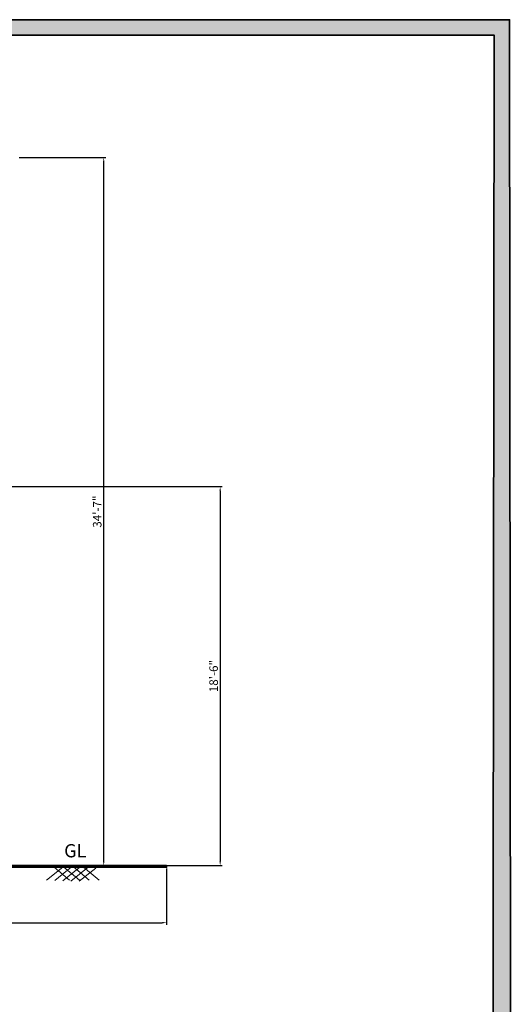
# Model space of a CAD drawing. Units: inches. Extents: x 1804 to 3296, y 909 to 2477.
# Tile 31 of 31: x 3008 to 3296, y 1900 to 2477. Entities that reach past the tile are written whole.
import ezdxf

# ---------------------------------------------------------------- set-up
doc = ezdxf.new("R2010")
doc.units = ezdxf.units.IN
for name, color, linetype, lineweight in [('A-ANNO-DIMS', 2, 'Continuous', 18), ('A-ANNO-TTLB', 156, 'Continuous', 35), ('A-SECT-PATT', 160, 'Continuous', 13), ('A-WALL-PATT', 10, 'Continuous', 13), ('C-GRAD-PATT', 8, 'Continuous', 13), ('SEC', 160, 'Continuous', 35), ('TEXT', 190, 'Continuous', 18)]:
    doc.layers.add(name, color=color, linetype=linetype, lineweight=lineweight)
doc.styles.get("Standard").update_dxf_attribs({"font": 'arial.ttf'})
doc.dimstyles.new('ISO-25', dxfattribs={"dimtxt": 5, "dimasz": 2.5, "dimexe": 1.25, "dimexo": 0.625, "dimtad": 1, "dimdec": 0, "dimlunit": 4, "dimtxsty": 'Standard', "dimcen": 2.5, "dimadec": 0, "dimazin": 0, "dimtfac": 1, "dimtdec": 0, "dimtmove": 0, "dimatfit": 3, "dimfxl": 1, "dimarcsym": 0})

# ---------------------------------------------------------------- blocks, each defined once
blk = doc.blocks.new('*D33')
at = {"layer": 'A-ANNO-DIMS', "color": 0, "lineweight": -2, "transparency": 16777216}
for p, q in [((3007.45, 2395.8), (3058.21, 2395.8)), ((3056.96, 1983.77), (3056.96, 2393.3)), ((3007.45, 1981.27), (3058.21, 1981.27))]:
    blk.add_line(p, q, dxfattribs=at)
at = {"layer": 'A-ANNO-DIMS', "color": 0, "lineweight": 100, "transparency": 16777216}
for points in [[(3056.55, 2393.3), (3057.38, 2393.3), (3056.96, 2395.8)], [(3056.55, 1983.77), (3057.38, 1983.77), (3056.96, 1981.27)]]:
    blk.add_solid(points, dxfattribs=at)
at = {"layer": 'Defpoints', "color": 0, "lineweight": 100, "transparency": 16777216}
for p in [(3006.82, 2395.8), (3056.96, 2395.8), (3006.82, 1981.27)]:
    blk.add_point(p, dxfattribs=at)
at = {"layer": 'A-ANNO-DIMS', "color": 0, "transparency": 16777216, "insert": (3053.79, 2188.53), "char_height": 5, "attachment_point": 5, "rotation": 90}
blk.add_mtext('34\'-7"', dxfattribs=at)
blk = doc.blocks.new('*D91')
at = {"layer": 'A-ANNO-DIMS', "color": 0, "lineweight": -2, "transparency": 16777216}
for p, q in [((2490.75, 1978.65), (2490.75, 1946.62)), ((3093.73, 1979.65), (3093.73, 1946.62)), ((2493.25, 1947.87), (3091.23, 1947.87))]:
    blk.add_line(p, q, dxfattribs=at)
at = {"layer": 'A-ANNO-DIMS', "color": 0, "lineweight": 100, "transparency": 16777216}
for points in [[(2493.25, 1948.29), (2493.25, 1947.46), (2490.75, 1947.87)], [(3091.23, 1948.29), (3091.23, 1947.46), (3093.73, 1947.87)]]:
    blk.add_solid(points, dxfattribs=at)
at = {"layer": 'Defpoints', "color": 0, "lineweight": 100, "transparency": 16777216}
for p in [(2490.75, 1979.27), (3093.73, 1980.27), (3093.73, 1947.87)]:
    blk.add_point(p, dxfattribs=at)
at = {"layer": 'A-ANNO-DIMS', "color": 0, "transparency": 16777216, "insert": (2792.24, 1951.05), "char_height": 5, "attachment_point": 5}
blk.add_mtext('50\'-3"', dxfattribs=at)
blk = doc.blocks.new('*D93')
at = {"layer": 'A-ANNO-DIMS', "color": 0, "lineweight": -2, "transparency": 16777216}
for p, q in [((2997.45, 2203.2), (3126.38, 2203.2)), ((3125.13, 2200.7), (3125.13, 1983.77)), ((3007.45, 1981.27), (3126.38, 1981.27))]:
    blk.add_line(p, q, dxfattribs=at)
at = {"layer": 'A-ANNO-DIMS', "color": 0, "lineweight": 100, "transparency": 16777216}
for points in [[(3124.71, 2200.7), (3125.55, 2200.7), (3125.13, 2203.2)], [(3124.71, 1983.77), (3125.55, 1983.77), (3125.13, 1981.27)]]:
    blk.add_solid(points, dxfattribs=at)
at = {"layer": 'Defpoints', "color": 0, "lineweight": 100, "transparency": 16777216}
for p in [(2996.82, 2203.2), (3006.82, 1981.27), (3125.13, 1981.27)]:
    blk.add_point(p, dxfattribs=at)
at = {"layer": 'A-ANNO-DIMS', "color": 0, "transparency": 16777216, "insert": (3121.95, 2092.24), "char_height": 5, "attachment_point": 5, "rotation": 90}
blk.add_mtext('18\'-6"', dxfattribs=at)

msp = doc.modelspace()

# ---------------------------------------------------------------- hatches: boundary and pattern name
at = {"layer": 'A-ANNO-TTLB'}
h = msp.add_hatch(color=256, dxfattribs=at)
h.dxf.hatch_style = 1
h.paths.add_polyline_path([(3294.53, 2476.54), (1803.79, 2476.54), (1805.43, 909.47), (3296.17, 909.47)])
h.paths.add_polyline_path([(1811, 914.33), (1812.79, 2467.54), (3285.53, 2467.54), (3283.74, 914.33)], flags=16)
h.paths.add_polyline_path([(1925.58, 1062.77), (1925.58, 1138.07), (1925.58, 1539.88), (1925.58, 1793.38), (1925.58, 1830.04), (2325.54, 1830.04), (2325.54, 1793.38), (2325.54, 1586.42), (2325.54, 1138.07), (2325.54, 1062.77)], flags=0)
h.paths.add_polyline_path([(1997.22, 1029.4), (2008.85, 1037.96), (2008.85, 1020.84)], flags=0)
h.paths.add_polyline_path([(1934.58, 1138.07), (1934.58, 1147.07), (2078.77, 1147.07), (2078.77, 1138.07), (2060.94, 1138.07)], flags=0)
h.paths.add_polyline_path([(1944.35, 1138.07), (1944.35, 1147.07), (2056.05, 1147.07), (2056.05, 1138.07)], flags=0)
h.paths.add_polyline_path([(2222.24, 1037.96), (2233.87, 1029.4), (2222.24, 1020.84)], flags=0)
h.paths.add_polyline_path([(2061.94, 1139.07), (2061.94, 1146.07), (2077.77, 1146.07), (2077.77, 1139.07)], flags=0)
h.paths.add_polyline_path([(2149.58, 1138.07), (2149.58, 1269.44), (2158.58, 1269.44), (2158.58, 1326.69), (2149.58, 1326.69), (2149.58, 1340.94), (2139.6, 1340.94), (2139.6, 1434.25), (2149.58, 1434.25), (2149.58, 1447.36), (2158.58, 1447.36), (2158.58, 1423.87), (2158.58, 1408.06), (2198.46, 1408.06), (2198.46, 1412.56), (2282.65, 1412.56), (2282.65, 1465.94), (2316.54, 1465.94), (2316.54, 1590.92), (2192.86, 1590.92), (2192.86, 1595.3), (2291.17, 1595.3), (2291.17, 1590.92), (2316.54, 1590.92), (2316.54, 1784.38), (2300.24, 1784.38), (2300.24, 1757.47), (2268, 1757.47), (2268, 1681.04), (2180.87, 1681.04), (2180.87, 1757.47), (2148.63, 1757.47), (2148.63, 1784.38), (2119.08, 1784.38), (2119.08, 1585.58), (2114.58, 1585.58), (2114.58, 1784.38), (2064.11, 1784.38), (2046.28, 1784.38), (2046.28, 1760.38), (1958.58, 1760.38), (1958.58, 1664.38), (1934.58, 1664.38), (1934.58, 1784.38), (1934.58, 1793.38), (2046.28, 1793.38), (2064.11, 1793.38), (2119.08, 1793.38), (2230.78, 1793.38), (2230.78, 1784.38), (2268, 1784.38), (2300.24, 1784.38), (2316.54, 1784.38), (2316.54, 1590.92), (2316.54, 1373.73), (2316.54, 1138.07)], flags=0)
h.paths.add_polyline_path([(2209.19, 1166.63), (2209.19, 1175.63), (2158.58, 1175.63), (2209.19, 1223.63), (2209.19, 1231.63), (2183.88, 1231.63), (2183.88, 1301.66), (2242.59, 1301.66), (2242.59, 1326.69), (2316.54, 1326.69), (2272.59, 1271.63), (2272.59, 1223.63), (2316.54, 1175.63), (2272.59, 1175.63), (2272.59, 1166.63)], flags=0)
h.paths.add_polyline_path([(1947.77, 1345.22), (1947.77, 1457.48), (1991.2, 1457.48), (1991.2, 1451.7), (1991.2, 1352.18), (1991.2, 1345.22)], flags=0)
h.paths.add_polyline_path([(2209.19, 1271.63), (2262.59, 1271.63), (2262.59, 1311.85), (2272.59, 1301.66), (2272.59, 1271.63), (2269.92, 1269.63), (2270.59, 1269.63), (2270.59, 1225.63), (2211.19, 1225.63), (2211.19, 1269.63), (2211.86, 1269.63)], flags=0)
h.paths.add_polyline_path([(2000.34, 1378.21), (2000.34, 1429.71), (2025.22, 1429.71), (2025.22, 1378.21)], flags=0)
h.paths.add_polyline_path([(2001.34, 1379.21), (2001.34, 1428.71), (2024.22, 1428.71), (2024.22, 1379.21)], flags=0)
h.paths.add_polyline_path([(2012.34, 1390.21), (2012.34, 1417.71), (2013.22, 1417.71), (2013.22, 1390.21)], flags=0)
h.paths.add_polyline_path([(2237.56, 1331.19), (2237.56, 1340.18), (2238.62, 1340.18), (2238.62, 1386.84), (2241.04, 1386.84), (2242.06, 1386.84), (2242.06, 1408.06), (2316.54, 1331.19)], flags=0)
h.paths.add_polyline_path([(1953.73, 1464.35), (1953.73, 1498.59), (1981.74, 1498.59), (1981.74, 1464.35)], flags=0)
h.paths.add_polyline_path([(1987.63, 1462.08), (1987.63, 1500.95), (2104.07, 1500.95), (2104.07, 1462.08), (2099.27, 1462.08), (1993.6, 1462.08)], flags=0)
h.paths.add_polyline_path([(1956.06, 1481.47, -1), (1979.41, 1481.47, -1)], flags=0)
edge = h.paths.add_edge_path(flags=0)
edge.add_ellipse((2299.53, 1438.37), major_axis=(0.31, 21.36), ratio=0.670333, start_angle=0, end_angle=360)
h.paths.add_polyline_path([(2297.39, 1438.37, -1), (2301.67, 1438.37, -1)], flags=0)
h.paths.add_polyline_path([(2591.54, 1163.23), (2591.54, 1179.38), (2591.54, 1379.68), (2591.54, 1395.84), (2734.5, 1395.84), (2734.5, 1379.68), (2734.5, 1179.38), (2734.5, 1163.23)], flags=0)
h.paths.add_polyline_path([(2592.54, 1164.23), (2592.54, 1166.23), (2733.5, 1166.23), (2733.5, 1164.23)], flags=0)
h.paths.add_polyline_path([(2592.54, 1180.38), (2592.54, 1378.68), (2733.5, 1378.68), (2733.5, 1180.38)], flags=0)
h.paths.add_polyline_path([(2593.54, 1181.38), (2593.54, 1377.68), (2732.5, 1377.68), (2732.5, 1181.38)], flags=0)
h.paths.add_polyline_path([(2594.54, 1182.38), (2594.54, 1376.68), (2731.5, 1376.68), (2731.5, 1182.38)], flags=0)
h.paths.add_polyline_path([(1936.95, 1697.46), (1936.95, 1736.46), (1955.41, 1736.46), (1955.41, 1697.46)], flags=0)
h.paths.add_polyline_path([(1938.48, 1718.36), (1938.48, 1734.92), (1953.65, 1734.92), (1953.65, 1718.36)], flags=0)
h.paths.add_polyline_path([(1944.75, 1726.64, -1), (1947.37, 1726.64, -1)], flags=0)
h.paths.add_polyline_path([(2592.54, 1394.84), (2733.5, 1394.84), (2733.5, 1392.84), (2592.54, 1392.84)], flags=0)
h.paths.add_polyline_path([(1976.61, 1762.5), (1976.61, 1781.44), (2012.79, 1781.44), (2012.79, 1762.5)], flags=0)
h.paths.add_polyline_path([(1979.57, 1771.97, -1), (1991.39, 1771.97, -1)], flags=0)
h.paths.add_polyline_path([(1995.36, 1771.97, -1), (2007.18, 1771.97, -1)], flags=0)
h.paths.add_polyline_path([(2251.51, 1744.53), (2268, 1730.05), (2251.51, 1730.05)], flags=0)
h.paths.add_polyline_path([(2047.28, 1785.38), (2047.28, 1792.38), (2063.11, 1792.38), (2063.11, 1785.38)], flags=0)
h.paths.add_polyline_path([(2155.08, 1770.92, -1), (2174.42, 1770.92, -1)], flags=0)
h.paths.add_polyline_path([(2188.59, 1758.27), (2188.59, 1772.81), (2222.3, 1772.81), (2222.3, 1758.27)], flags=0)
h.paths.add_polyline_path([(2223.97, 1758.27), (2223.97, 1772.81), (2257.68, 1772.81), (2257.68, 1758.27)], flags=0)
h.paths.add_polyline_path([(2274.45, 1770.92, -1), (2293.8, 1770.92, -1)], flags=0)
h.paths.add_polyline_path([(2591.54, 1582.09), (2591.54, 1782.39), (2734.5, 1782.39), (2734.5, 1582.09)], flags=0)
h.paths.add_polyline_path([(2592.54, 1583.09), (2592.54, 1781.39), (2733.5, 1781.39), (2733.5, 1583.09)], flags=0)
h.paths.add_polyline_path([(2593.54, 1584.09), (2593.54, 1780.39), (2732.5, 1780.39), (2732.5, 1584.09)], flags=0)
h.paths.add_polyline_path([(2594.54, 1585.09), (2594.54, 1779.39), (2731.5, 1779.39), (2731.5, 1585.09)], flags=0)
h.paths.add_polyline_path([(1922.17, 1978.79), (1922.17, 2295.08), (1922.17, 2296.08), (2115.67, 2296.08), (2115.67, 2384.31), (2115.67, 2385.31), (2322.12, 2385.31), (2323.12, 2385.31), (2323.12, 1979.79), (2323.12, 1978.79), (1923.17, 1978.79)], flags=0)
h.paths.add_polyline_path([(1922.17, 1978.79), (1922.17, 2051.31), (1922.17, 2214.86), (1922.17, 2296.08), (2115.67, 2296.08), (2115.67, 2385.31), (2323.12, 2385.31), (2323.12, 2280.42), (2323.12, 1978.79), (2115.67, 1978.79)], flags=0)
h.paths.add_polyline_path([(1923.17, 1979.79), (1923.17, 2050.31), (2115.67, 2050.31), (2115.67, 2051.31), (1923.17, 2051.31), (1923.17, 2213.86), (1923.17, 2214.86), (1923.17, 2295.08), (1990.02, 2295.08), (1990.02, 2214.86), (1991.02, 2214.86), (1991.02, 2295.08), (2115.67, 2295.08), (2115.67, 1979.79), (2116.67, 1979.79), (2116.67, 2304.18), (2116.67, 2384.31), (2322.12, 2384.31), (2322.12, 2280.42), (2322.12, 1979.79), (2115.67, 1979.79)], flags=0)
h.paths.add_polyline_path([(2972.46, 1192.5), (2972.46, 1196.92), (2995.47, 1196.92), (2995.47, 1255.47), (2995.09, 1255.47), (2987.42, 1249.39), (2980.08, 1255.47), (2978.05, 1255.47), (2978.05, 1257.24), (2995.47, 1257.24), (2995.47, 1261.58), (3015.37, 1261.58), (3015.37, 1333.28), (3015.37, 1414.4), (3032.82, 1414.4), (3032.82, 1333.28), (3032.82, 1261.58), (3052.66, 1261.58), (3052.66, 1255.47), (3079.86, 1255.47), (3078.72, 1254.57), (3081.47, 1252.29), (3078.56, 1249.99), (3075.81, 1252.26), (3072.57, 1249.69), (3070.36, 1251.52), (3067.67, 1249.39), (3060.34, 1255.47), (3052.66, 1255.47), (3052.66, 1196.92), (3054.58, 1196.92), (3074, 1196.92), (3074, 1192.5), (3052.66, 1192.5), (2995.47, 1192.5)], flags=0)
h.paths.add_polyline_path([(2490.75, 1979.27), (2490.75, 1980.27), (2596.87, 1980.27), (2596.87, 2051.8), (2596.87, 2052.8), (2596.87, 2216.35), (2596.87, 2297.57), (2717.32, 2297.57), (2710.57, 2305.62), (2724.07, 2305.62), (2717.32, 2297.57), (2782.37, 2297.57), (2782.37, 2395.8), (3006.82, 2395.8), (3006.82, 1981.27), (3093.73, 1981.27), (3093.73, 1980.27), (3047.51, 1980.27), (3046.37, 1979.37), (3049.11, 1977.1), (3046.2, 1974.79), (3043.46, 1977.07), (3040.21, 1974.49), (3038, 1976.32), (3035.32, 1974.2), (3027.98, 1980.27), (2871.83, 1980.27), (2871.83, 1981.27), (2791.37, 1981.27), (2791.37, 2050.8), (2597.87, 2050.8), (2597.87, 1980.27), (2597.87, 1979.27), (2546.27, 1979.27), (2545.12, 1978.37), (2547.87, 1976.1), (2544.96, 1973.79), (2542.22, 1976.07), (2538.97, 1973.49), (2536.76, 1975.32), (2534.07, 1973.2), (2526.74, 1979.27)], flags=0)
h.paths.add_polyline_path([(2597.87, 2051.8), (2606.87, 2051.8), (2606.87, 2258.39), (2597.87, 2258.39), (2597.87, 2296.57), (2606.87, 2296.57), (2606.87, 2262.39), (2782.37, 2262.39), (2782.37, 2296.57), (2790.37, 2296.57), (2790.37, 2262.39), (2791.37, 2262.39), (2791.37, 2305.67), (2791.37, 2385.8), (2996.82, 2385.8), (2996.82, 2339.85), (3006.82, 2339.85), (3006.82, 2250.12), (2997.82, 2250.12), (2997.82, 1981.27), (2996.82, 1981.27), (2872.83, 1981.27), (2872.83, 1991.8), (2871.83, 1991.8), (2871.83, 2050.8), (2790.37, 2050.8), (2597.87, 2050.8)], flags=0)
h.paths.add_polyline_path([(2179.93, 2153.92), (2179.93, 2353.97), (2259.98, 2353.97), (2259.98, 2153.92)], flags=0)
h.paths.add_polyline_path([(2180.93, 2154.92), (2180.93, 2352.97), (2258.98, 2352.97), (2258.98, 2154.92)], flags=0)
h.paths.add_polyline_path([(2960.87, 1608.49), (2960.87, 1753.62), (3070.9, 1753.62), (3070.9, 1608.49)], flags=0)
h.paths.add_polyline_path([(2961.87, 1609.49), (2961.87, 1752.62), (3069.9, 1752.62), (3069.9, 1609.49)], flags=0)
h.paths.add_polyline_path([(2962.87, 1610.49), (2962.87, 1751.62), (3068.9, 1751.62), (3068.9, 1610.49)], flags=0)
h.paths.add_polyline_path([(2963.87, 1611.49), (2963.87, 1750.62), (3067.9, 1750.62), (3067.9, 1611.49)], flags=0)
h.paths.add_polyline_path([(2782.37, 2051.8), (2782.37, 2216.32), (2791.37, 2216.32), (2791.37, 2051.8), (2872.83, 2051.8), (2872.83, 2068.56), (2884.67, 2068.56), (2884.67, 2085.33), (2896.51, 2085.33), (2896.51, 2102.09), (2908.36, 2102.09), (2908.36, 2118.85), (2920.2, 2118.85), (2920.2, 2135.62), (2932.05, 2135.62), (2932.05, 2145.3), (2925.08, 2145.3), (2925.08, 2203.2), (2996.82, 2203.2), (2996.82, 2145.3), (2953.82, 2145.3), (2872.83, 2051.8), (2790.37, 2051.8)], flags=0)
h.paths.add_polyline_path([(2717.32, 2238.65), (2710.57, 2246.7), (2724.07, 2246.7)], flags=0)
h.paths.add_polyline_path([(2003.09, 1122.79), (2017.16, 1122.79), (2017.16, 1138.74), (2003.09, 1138.74)], flags=8)
h.paths.add_polyline_path([(2174.76, 1792.72), (2188.83, 1792.72), (2188.83, 1808.66), (2174.76, 1808.66)], flags=8)
h.paths.add_polyline_path([(1987.95, 1792.51), (2002.02, 1792.51), (2002.02, 1808.45), (1987.95, 1808.45)], flags=8)
h.paths.add_polyline_path([(2148.79, 1289.26), (2160.46, 1289.26), (2160.46, 1305.2), (2148.79, 1305.2)], flags=8)
h.paths.add_polyline_path([(2115.36, 1133.57), (2127.04, 1133.57), (2127.04, 1149.51), (2115.36, 1149.51)], flags=8)
h.paths.add_polyline_path([(2237.58, 1421.48), (2249.25, 1421.48), (2249.25, 1437.43), (2237.58, 1437.43)], flags=8)
h.paths.add_polyline_path([(2134.99, 1584.32), (2146.66, 1584.32), (2146.66, 1600.26), (2134.99, 1600.26)], flags=8)
h.paths.add_polyline_path([(2101.95, 1557.31), (2113.62, 1557.31), (2113.62, 1573.25), (2101.95, 1573.25)], flags=8)
h.paths.add_polyline_path([(2937.85, 1156.77), (3120.41, 1156.77), (3120.41, 1185.72), (2937.85, 1185.72)], flags=8)
h.paths.add_polyline_path([(2980.71, 1786.71), (3050.06, 1786.71), (3050.06, 1802.66), (2980.71, 1802.66)], flags=8)
h.paths.add_polyline_path([(2869.28, 1661.96), (2938.62, 1661.96), (2938.62, 1690.8), (2869.28, 1690.8)], flags=8)
h.paths.add_polyline_path([(3092.27, 1674.86), (3161.62, 1674.86), (3161.62, 1690.8), (3092.27, 1690.8)], flags=8)
h.paths.add_polyline_path([(2980.71, 1674.86), (3050.06, 1674.86), (3050.06, 1690.8), (2980.71, 1690.8)], flags=8)
h.paths.add_polyline_path([(2649.07, 1678.23), (2674.53, 1678.23), (2674.53, 1714.76), (2649.07, 1714.76)], flags=8)
h.paths.add_polyline_path([(2530.84, 1981.63), (2549.13, 1981.63), (2549.13, 1997.57), (2530.84, 1997.57)], flags=8)
h.paths.add_polyline_path([(3031.29, 1981.77), (3049.58, 1981.77), (3049.58, 1997.71), (3031.29, 1997.71)], flags=8)
h.paths.add_polyline_path([(2715.38, 1911.9), (2851.54, 1911.9), (2851.54, 1940.85), (2715.38, 1940.85)], flags=8)
h.paths.add_polyline_path([(2015.23, 1927.36), (2205.42, 1927.36), (2205.42, 1956.3), (2015.23, 1956.3)], flags=8)
h.paths.add_polyline_path([(2671.84, 2057.84), (2702.75, 2057.84), (2702.75, 2073.79), (2671.84, 2073.79)], flags=8)
h.paths.add_polyline_path([(2678.5, 2316.52), (2765.26, 2316.52), (2765.26, 2332.46), (2678.5, 2332.46)], flags=8)
h.paths.add_polyline_path([(2678.48, 2271.96), (2736.41, 2271.96), (2736.41, 2287.9), (2678.48, 2287.9)], flags=8)
h.paths.add_polyline_path([(2019.2, 972.79), (2243.21, 972.79), (2243.21, 1001.74), (2019.2, 1001.74)], flags=8)
h.paths.add_polyline_path([(2097.06, 1021.56), (2132.16, 1021.56), (2132.16, 1037.51), (2097.06, 1037.51)], flags=8)
h.paths.add_polyline_path([(2182.47, 1360.48), (2207.35, 1360.48), (2207.35, 1376.42), (2182.47, 1376.42)], flags=8)
h.paths.add_polyline_path([(2261.12, 1361.77), (2295.01, 1361.77), (2295.01, 1377.71), (2261.12, 1377.71)], flags=8)
h.paths.add_polyline_path([(2245.75, 1511.51), (2278.44, 1511.51), (2278.44, 1527.46), (2245.75, 1527.46)], flags=8)
h.paths.add_polyline_path([(1991.16, 1296.29), (2060.51, 1296.29), (2060.51, 1312.23), (1991.16, 1312.23)], flags=8)
h.paths.add_polyline_path([(2187, 1651.35), (2246.71, 1651.35), (2246.71, 1667.29), (2187, 1667.29)], flags=8)
h.paths.add_polyline_path([(1976.49, 1684.81), (2068.63, 1684.81), (2068.63, 1700.76), (1976.49, 1700.76)], flags=8)
at = {"layer": 'A-SECT-PATT'}
h = msp.add_hatch(color=256, dxfattribs=at)
h.dxf.hatch_style = 1
h.paths.add_polyline_path([(3093.73, 1981.27), (2871.83, 1981.27), (2871.83, 1980.27), (3093.73, 1980.27)])
at = {"layer": 'A-WALL-PATT'}
h = msp.add_hatch(color=256, dxfattribs=at)
h.dxf.hatch_style = 1
h.paths.add_polyline_path([(2119.08, 1544.38), (1925.58, 1544.38), (1925.58, 1539.88), (2119.08, 1539.88)])
h.paths.add_polyline_path([(2119.08, 1545.58), (2114.58, 1545.58), (2114.58, 1544.38), (2119.08, 1544.38)])
h.paths.add_polyline_path([(1965.87, 1658.79), (1965.87, 1679.09), (1955.57, 1679.09), (1955.57, 1658.79)], flags=9)
h.paths.add_polyline_path([(2293.18, 1677.29), (2293.18, 1697.58), (2282.88, 1697.58), (2282.88, 1677.29)], flags=9)
h.paths.add_polyline_path([(2271.13, 1545.23), (2287.53, 1545.23), (2287.53, 1555.53), (2271.13, 1555.53)], flags=9)
h.paths.add_polyline_path([(2303.26, 1488.52), (2303.26, 1508.82), (2292.95, 1508.82), (2292.95, 1488.52)], flags=9)
h.paths.add_polyline_path([(2271.13, 1393.15), (2287.53, 1393.15), (2287.53, 1403.45), (2271.13, 1403.45)], flags=9)
h.paths.add_polyline_path([(2306.48, 1361.45), (2306.48, 1377.86), (2296.18, 1377.86), (2296.18, 1361.45)], flags=9)
h.paths.add_polyline_path([(2174.54, 1361.45), (2174.54, 1377.86), (2164.23, 1377.86), (2164.23, 1361.45)], flags=9)
h.paths.add_polyline_path([(1968.21, 1333.34), (1968.21, 1353.64), (1957.91, 1353.64), (1957.91, 1333.34)], flags=9)
h.paths.add_polyline_path([(2003.09, 1122.79), (2017.16, 1122.79), (2017.16, 1138.74), (2003.09, 1138.74)], flags=9)
h.paths.add_polyline_path([(2174.76, 1792.72), (2188.83, 1792.72), (2188.83, 1808.66), (2174.76, 1808.66)], flags=9)
h.paths.add_polyline_path([(1987.95, 1792.51), (2002.02, 1792.51), (2002.02, 1808.45), (1987.95, 1808.45)], flags=9)
h.paths.add_polyline_path([(2148.79, 1289.26), (2160.46, 1289.26), (2160.46, 1305.2), (2148.79, 1305.2)], flags=9)
h.paths.add_polyline_path([(2115.36, 1133.57), (2127.04, 1133.57), (2127.04, 1149.51), (2115.36, 1149.51)], flags=9)
h.paths.add_polyline_path([(2237.58, 1421.48), (2249.25, 1421.48), (2249.25, 1437.43), (2237.58, 1437.43)], flags=9)
h.paths.add_polyline_path([(2134.99, 1584.32), (2146.66, 1584.32), (2146.66, 1600.26), (2134.99, 1600.26)], flags=9)
h.paths.add_polyline_path([(2101.95, 1557.31), (2113.62, 1557.31), (2113.62, 1573.25), (2101.95, 1573.25)], flags=9)
h.paths.add_polyline_path([(2937.85, 1156.77), (3120.41, 1156.77), (3120.41, 1185.72), (2937.85, 1185.72)], flags=9)
h.paths.add_polyline_path([(2980.71, 1786.71), (3050.06, 1786.71), (3050.06, 1802.66), (2980.71, 1802.66)], flags=9)
h.paths.add_polyline_path([(2869.28, 1661.96), (2938.62, 1661.96), (2938.62, 1690.8), (2869.28, 1690.8)], flags=9)
h.paths.add_polyline_path([(3092.27, 1674.86), (3161.62, 1674.86), (3161.62, 1690.8), (3092.27, 1690.8)], flags=9)
h.paths.add_polyline_path([(2980.71, 1674.86), (3050.06, 1674.86), (3050.06, 1690.8), (2980.71, 1690.8)], flags=9)
h.paths.add_polyline_path([(2649.07, 1678.23), (2674.53, 1678.23), (2674.53, 1714.76), (2649.07, 1714.76)], flags=9)
h.paths.add_polyline_path([(2530.84, 1981.63), (2549.13, 1981.63), (2549.13, 1997.57), (2530.84, 1997.57)], flags=9)
h.paths.add_polyline_path([(3031.29, 1981.77), (3049.58, 1981.77), (3049.58, 1997.71), (3031.29, 1997.71)], flags=9)
h.paths.add_polyline_path([(2715.38, 1911.9), (2851.54, 1911.9), (2851.54, 1940.85), (2715.38, 1940.85)], flags=9)
h.paths.add_polyline_path([(2015.23, 1927.36), (2205.42, 1927.36), (2205.42, 1956.3), (2015.23, 1956.3)], flags=9)
h.paths.add_polyline_path([(2671.84, 2057.84), (2702.75, 2057.84), (2702.75, 2073.79), (2671.84, 2073.79)], flags=9)
h.paths.add_polyline_path([(2678.5, 2316.52), (2765.26, 2316.52), (2765.26, 2332.46), (2678.5, 2332.46)], flags=9)
h.paths.add_polyline_path([(2678.48, 2271.96), (2736.41, 2271.96), (2736.41, 2287.9), (2678.48, 2287.9)], flags=9)
h.paths.add_polyline_path([(2019.2, 972.79), (2243.21, 972.79), (2243.21, 1001.74), (2019.2, 1001.74)], flags=9)
h.paths.add_polyline_path([(2097.06, 1021.56), (2132.16, 1021.56), (2132.16, 1037.51), (2097.06, 1037.51)], flags=9)
h.paths.add_polyline_path([(2182.47, 1360.48), (2207.35, 1360.48), (2207.35, 1376.42), (2182.47, 1376.42)], flags=9)
h.paths.add_polyline_path([(2261.12, 1361.77), (2295.01, 1361.77), (2295.01, 1377.71), (2261.12, 1377.71)], flags=9)
h.paths.add_polyline_path([(2245.75, 1511.51), (2278.44, 1511.51), (2278.44, 1527.46), (2245.75, 1527.46)], flags=9)
h.paths.add_polyline_path([(1991.16, 1296.29), (2060.51, 1296.29), (2060.51, 1312.23), (1991.16, 1312.23)], flags=9)
h.paths.add_polyline_path([(2187, 1651.35), (2246.71, 1651.35), (2246.71, 1667.29), (2187, 1667.29)], flags=9)
h.paths.add_polyline_path([(1976.49, 1684.81), (2068.63, 1684.81), (2068.63, 1700.76), (1976.49, 1700.76)], flags=9)
h = msp.add_hatch(color=256, dxfattribs=at)
h.dxf.hatch_style = 1
h.paths.add_polyline_path([(2149.58, 1147.07), (2141.21, 1147.07), (2141.21, 1144.07), (2141.21, 1138.07), (2149.58, 1138.07)])
h.paths.add_polyline_path([(2101.21, 1144.07, -0.01877), (2101.32, 1147.07), (2078.77, 1147.07), (2078.77, 1138.07), (2101.21, 1138.07)])
h.paths.add_polyline_path([(2060.94, 1147.07), (2056.05, 1147.07), (2056.05, 1138.07), (2060.94, 1138.07)])
h.paths.add_polyline_path([(1944.35, 1147.07), (1934.58, 1147.07), (1934.58, 1138.07), (1944.35, 1138.07)])
h.paths.add_polyline_path([(2158.58, 1269.44), (2149.58, 1269.44), (2149.58, 1138.07), (2158.58, 1138.07)])
h.paths.add_polyline_path([(2003.09, 1122.79), (2017.16, 1122.79), (2017.16, 1138.74), (2003.09, 1138.74)], flags=9)
h.paths.add_polyline_path([(2174.76, 1792.72), (2188.83, 1792.72), (2188.83, 1808.66), (2174.76, 1808.66)], flags=9)
h.paths.add_polyline_path([(1987.95, 1792.51), (2002.02, 1792.51), (2002.02, 1808.45), (1987.95, 1808.45)], flags=9)
h.paths.add_polyline_path([(2148.79, 1289.26), (2160.46, 1289.26), (2160.46, 1305.2), (2148.79, 1305.2)], flags=9)
h.paths.add_polyline_path([(2115.36, 1133.57), (2127.04, 1133.57), (2127.04, 1149.51), (2115.36, 1149.51)], flags=9)
h.paths.add_polyline_path([(2237.58, 1421.48), (2249.25, 1421.48), (2249.25, 1437.43), (2237.58, 1437.43)], flags=9)
h.paths.add_polyline_path([(2134.99, 1584.32), (2146.66, 1584.32), (2146.66, 1600.26), (2134.99, 1600.26)], flags=9)
h.paths.add_polyline_path([(2101.95, 1557.31), (2113.62, 1557.31), (2113.62, 1573.25), (2101.95, 1573.25)], flags=9)
h.paths.add_polyline_path([(2937.85, 1156.77), (3120.41, 1156.77), (3120.41, 1185.72), (2937.85, 1185.72)], flags=9)
h.paths.add_polyline_path([(2980.71, 1786.71), (3050.06, 1786.71), (3050.06, 1802.66), (2980.71, 1802.66)], flags=9)
h.paths.add_polyline_path([(2869.28, 1661.96), (2938.62, 1661.96), (2938.62, 1690.8), (2869.28, 1690.8)], flags=9)
h.paths.add_polyline_path([(3092.27, 1674.86), (3161.62, 1674.86), (3161.62, 1690.8), (3092.27, 1690.8)], flags=9)
h.paths.add_polyline_path([(2980.71, 1674.86), (3050.06, 1674.86), (3050.06, 1690.8), (2980.71, 1690.8)], flags=9)
h.paths.add_polyline_path([(2649.07, 1678.23), (2674.53, 1678.23), (2674.53, 1714.76), (2649.07, 1714.76)], flags=9)
h.paths.add_polyline_path([(2530.84, 1981.63), (2549.13, 1981.63), (2549.13, 1997.57), (2530.84, 1997.57)], flags=9)
h.paths.add_polyline_path([(3031.29, 1981.77), (3049.58, 1981.77), (3049.58, 1997.71), (3031.29, 1997.71)], flags=9)
h.paths.add_polyline_path([(2715.38, 1911.9), (2851.54, 1911.9), (2851.54, 1940.85), (2715.38, 1940.85)], flags=9)
h.paths.add_polyline_path([(2015.23, 1927.36), (2205.42, 1927.36), (2205.42, 1956.3), (2015.23, 1956.3)], flags=9)
h.paths.add_polyline_path([(2671.84, 2057.84), (2702.75, 2057.84), (2702.75, 2073.79), (2671.84, 2073.79)], flags=9)
h.paths.add_polyline_path([(2678.5, 2316.52), (2765.26, 2316.52), (2765.26, 2332.46), (2678.5, 2332.46)], flags=9)
h.paths.add_polyline_path([(2678.48, 2271.96), (2736.41, 2271.96), (2736.41, 2287.9), (2678.48, 2287.9)], flags=9)
h.paths.add_polyline_path([(2019.2, 972.79), (2243.21, 972.79), (2243.21, 1001.74), (2019.2, 1001.74)], flags=9)
h.paths.add_polyline_path([(2097.06, 1021.56), (2132.16, 1021.56), (2132.16, 1037.51), (2097.06, 1037.51)], flags=9)
h.paths.add_polyline_path([(2182.47, 1360.48), (2207.35, 1360.48), (2207.35, 1376.42), (2182.47, 1376.42)], flags=9)
h.paths.add_polyline_path([(2261.12, 1361.77), (2295.01, 1361.77), (2295.01, 1377.71), (2261.12, 1377.71)], flags=9)
h.paths.add_polyline_path([(2245.75, 1511.51), (2278.44, 1511.51), (2278.44, 1527.46), (2245.75, 1527.46)], flags=9)
h.paths.add_polyline_path([(1991.16, 1296.29), (2060.51, 1296.29), (2060.51, 1312.23), (1991.16, 1312.23)], flags=9)
h.paths.add_polyline_path([(2187, 1651.35), (2246.71, 1651.35), (2246.71, 1667.29), (2187, 1667.29)], flags=9)
h.paths.add_polyline_path([(1976.49, 1684.81), (2068.63, 1684.81), (2068.63, 1700.76), (1976.49, 1700.76)], flags=9)
h = msp.add_hatch(color=256, dxfattribs=at)
h.dxf.hatch_style = 1
h.paths.add_polyline_path([(2158.58, 1275.49), (2155.29, 1275.49), (2149.58, 1275.49), (2149.58, 1269.44), (2158.58, 1269.44)])
h.paths.add_polyline_path([(2158.58, 1326.69), (2149.58, 1326.69), (2149.58, 1319.33), (2155.29, 1319.33), (2158.58, 1319.33)])
h.paths.add_polyline_path([(2158.58, 1402.2), (2158.58, 1423.87), (2158.58, 1447.36), (2149.58, 1447.36), (2149.58, 1423.87), (2149.58, 1340.94), (2149.58, 1326.69), (2158.58, 1326.69), (2158.58, 1354.23)])
h.paths.add_polyline_path([(1965.87, 1658.79), (1965.87, 1679.09), (1955.57, 1679.09), (1955.57, 1658.79)], flags=9)
h.paths.add_polyline_path([(2293.18, 1677.29), (2293.18, 1697.58), (2282.88, 1697.58), (2282.88, 1677.29)], flags=9)
h.paths.add_polyline_path([(2271.13, 1545.23), (2287.53, 1545.23), (2287.53, 1555.53), (2271.13, 1555.53)], flags=9)
h.paths.add_polyline_path([(2303.26, 1488.52), (2303.26, 1508.82), (2292.95, 1508.82), (2292.95, 1488.52)], flags=9)
h.paths.add_polyline_path([(2271.13, 1393.15), (2287.53, 1393.15), (2287.53, 1403.45), (2271.13, 1403.45)], flags=9)
h.paths.add_polyline_path([(2306.48, 1361.45), (2306.48, 1377.86), (2296.18, 1377.86), (2296.18, 1361.45)], flags=9)
h.paths.add_polyline_path([(2189.9, 1340.62), (2206.31, 1340.62), (2206.31, 1350.92), (2189.9, 1350.92)], flags=9)
h.paths.add_polyline_path([(2174.54, 1361.45), (2174.54, 1377.86), (2164.23, 1377.86), (2164.23, 1361.45)], flags=9)
h.paths.add_polyline_path([(2304.24, 1240.8), (2304.24, 1261.09), (2293.94, 1261.09), (2293.94, 1240.8)], flags=9)
h.paths.add_polyline_path([(2227.19, 1188.73), (2247.49, 1188.73), (2247.49, 1199.03), (2227.19, 1199.03)], flags=9)
h.paths.add_polyline_path([(2181.93, 1144.21), (2181.93, 1160.62), (2171.63, 1160.62), (2171.63, 1144.21)], flags=9)
h.paths.add_polyline_path([(1968.21, 1333.34), (1968.21, 1353.64), (1957.91, 1353.64), (1957.91, 1333.34)], flags=9)
h.paths.add_polyline_path([(2029.78, 1203.53), (2053.95, 1203.53), (2053.95, 1213.83), (2029.78, 1213.83)], flags=9)
h.paths.add_polyline_path([(2576.51, 1671.88), (2576.51, 1692.17), (2566.21, 1692.17), (2566.21, 1671.88)], flags=9)
h.paths.add_polyline_path([(2566.99, 1269.67), (2566.99, 1289.96), (2556.68, 1289.96), (2556.68, 1269.67)], flags=9)
h.paths.add_polyline_path([(2581.85, 1269.17), (2581.85, 1289.46), (2571.54, 1289.46), (2571.54, 1269.17)], flags=9)
h.paths.add_polyline_path([(2650.71, 1409.75), (2674.89, 1409.75), (2674.89, 1420.05), (2650.71, 1420.05)], flags=9)
h.paths.add_polyline_path([(2003.09, 1122.79), (2017.16, 1122.79), (2017.16, 1138.74), (2003.09, 1138.74)], flags=9)
h.paths.add_polyline_path([(2174.76, 1792.72), (2188.83, 1792.72), (2188.83, 1808.66), (2174.76, 1808.66)], flags=9)
h.paths.add_polyline_path([(1987.95, 1792.51), (2002.02, 1792.51), (2002.02, 1808.45), (1987.95, 1808.45)], flags=9)
h.paths.add_polyline_path([(2148.79, 1289.26), (2160.46, 1289.26), (2160.46, 1305.2), (2148.79, 1305.2)], flags=9)
h.paths.add_polyline_path([(2115.36, 1133.57), (2127.04, 1133.57), (2127.04, 1149.51), (2115.36, 1149.51)], flags=9)
h.paths.add_polyline_path([(2237.58, 1421.48), (2249.25, 1421.48), (2249.25, 1437.43), (2237.58, 1437.43)], flags=9)
h.paths.add_polyline_path([(2134.99, 1584.32), (2146.66, 1584.32), (2146.66, 1600.26), (2134.99, 1600.26)], flags=9)
h.paths.add_polyline_path([(2101.95, 1557.31), (2113.62, 1557.31), (2113.62, 1573.25), (2101.95, 1573.25)], flags=9)
h.paths.add_polyline_path([(2937.85, 1156.77), (3120.41, 1156.77), (3120.41, 1185.72), (2937.85, 1185.72)], flags=9)
h.paths.add_polyline_path([(2980.71, 1786.71), (3050.06, 1786.71), (3050.06, 1802.66), (2980.71, 1802.66)], flags=9)
h.paths.add_polyline_path([(2869.28, 1661.96), (2938.62, 1661.96), (2938.62, 1690.8), (2869.28, 1690.8)], flags=9)
h.paths.add_polyline_path([(3092.27, 1674.86), (3161.62, 1674.86), (3161.62, 1690.8), (3092.27, 1690.8)], flags=9)
h.paths.add_polyline_path([(2980.71, 1674.86), (3050.06, 1674.86), (3050.06, 1690.8), (2980.71, 1690.8)], flags=9)
h.paths.add_polyline_path([(2649.07, 1678.23), (2674.53, 1678.23), (2674.53, 1714.76), (2649.07, 1714.76)], flags=9)
h.paths.add_polyline_path([(2530.84, 1981.63), (2549.13, 1981.63), (2549.13, 1997.57), (2530.84, 1997.57)], flags=9)
h.paths.add_polyline_path([(3031.29, 1981.77), (3049.58, 1981.77), (3049.58, 1997.71), (3031.29, 1997.71)], flags=9)
h.paths.add_polyline_path([(2715.38, 1911.9), (2851.54, 1911.9), (2851.54, 1940.85), (2715.38, 1940.85)], flags=9)
h.paths.add_polyline_path([(2015.23, 1927.36), (2205.42, 1927.36), (2205.42, 1956.3), (2015.23, 1956.3)], flags=9)
h.paths.add_polyline_path([(2671.84, 2057.84), (2702.75, 2057.84), (2702.75, 2073.79), (2671.84, 2073.79)], flags=9)
h.paths.add_polyline_path([(2678.5, 2316.52), (2765.26, 2316.52), (2765.26, 2332.46), (2678.5, 2332.46)], flags=9)
h.paths.add_polyline_path([(2678.48, 2271.96), (2736.41, 2271.96), (2736.41, 2287.9), (2678.48, 2287.9)], flags=9)
h.paths.add_polyline_path([(2019.2, 972.79), (2243.21, 972.79), (2243.21, 1001.74), (2019.2, 1001.74)], flags=9)
h.paths.add_polyline_path([(2097.06, 1021.56), (2132.16, 1021.56), (2132.16, 1037.51), (2097.06, 1037.51)], flags=9)
h.paths.add_polyline_path([(2182.47, 1360.48), (2207.35, 1360.48), (2207.35, 1376.42), (2182.47, 1376.42)], flags=9)
h.paths.add_polyline_path([(2261.12, 1361.77), (2295.01, 1361.77), (2295.01, 1377.71), (2261.12, 1377.71)], flags=9)
h.paths.add_polyline_path([(2245.75, 1511.51), (2278.44, 1511.51), (2278.44, 1527.46), (2245.75, 1527.46)], flags=9)
h.paths.add_polyline_path([(1991.16, 1296.29), (2060.51, 1296.29), (2060.51, 1312.23), (1991.16, 1312.23)], flags=9)
h.paths.add_polyline_path([(2187, 1651.35), (2246.71, 1651.35), (2246.71, 1667.29), (2187, 1667.29)], flags=9)
h.paths.add_polyline_path([(1976.49, 1684.81), (2068.63, 1684.81), (2068.63, 1700.76), (1976.49, 1700.76)], flags=9)
at = {"layer": 'C-GRAD-PATT'}
h = msp.add_hatch(dxfattribs=at)
h.set_pattern_fill('ANSI31', color=256, scale=0.973088, angle=-6.62272, style=0)
h.paths.add_polyline_path([(3022.3, 1972.8), (3041.33, 1972.12), (3044.32, 1972.12), (3053.75, 1979.59), (3049, 1980.27), (3039.4, 1980.27), (3036.41, 1980.27), (3031.74, 1980.27)])
h = msp.add_hatch(dxfattribs=at)
h.set_pattern_fill('ANSI31', color=256, scale=1.158154, angle=95.36535, style=0)
h.paths.add_polyline_path([(3026.25, 1980.27), (3035.34, 1972.75), (3056.09, 1972.75), (3047.01, 1980.27)])

# ---------------------------------------------------------------- linework, layer by layer
at = {"layer": 'A-ANNO-TTLB'}
for points in [[(1803.79, 2476.54), (3294.53, 2476.54), (3296.17, 909.47), (1805.43, 909.47)], [(1812.79, 2467.54), (3285.53, 2467.54), (3283.74, 914.33), (1811, 914.33)]]:
    msp.add_lwpolyline(points, close=True, dxfattribs=at)
at = {"layer": 'SEC'}
for p, q in [((2996.82, 1981.27), (3093.73, 1981.27)), ((2996.82, 1980.27), (3093.73, 1980.27))]:
    msp.add_line(p, q, dxfattribs=at)
msp.add_lwpolyline([(2871.83, 1980.27), (3093.73, 1980.27), (3093.73, 1981.27), (2871.83, 1981.27)], close=True, dxfattribs=at)

# ---------------------------------------------------------------- texts
at = {"layer": 'TEXT', "insert": (3033.8, 1993.86), "char_height": 7.737, "attachment_point": 1}
msp.add_mtext_dynamic_manual_height_columns('GL', width=163.3261, gutter_width=38.69, heights=[0], dxfattribs=at)

# ---------------------------------------------------------------- dimensions: what is measured, and where the dimension line sits
at = {"layer": 'A-ANNO-DIMS'}
for base, p1, p2, override, picture, middle in [((3056.96, 2395.8), (3006.82, 1981.27), (3006.82, 2395.8), {"dimclrd": 0, "dimclre": 0, "dimclrt": 0}, '*D33', (3053.79, 2188.53)), ((3125.13, 1981.27), (2996.82, 2203.2), (3006.82, 1981.27), {"dimdec": 1, "dimlfac": 1, "dimrnd": 0, "dimzin": 1, "dimdsep": 46, "dimlunit": 4, "dimfrac": 2}, '*D93', (3121.95, 2092.24))]:
    dim = msp.add_linear_dim(base=base, p1=p1, p2=p2, angle=90, dimstyle='ISO-25', override=override, dxfattribs=at)
    dim.commit()
    dim.dimension.update_dxf_attribs({"geometry": picture, "text_midpoint": middle})
dim = msp.add_linear_dim(base=(3093.73, 1947.87), p1=(2490.75, 1979.27), p2=(3093.73, 1980.27), dimstyle='ISO-25', override={"dimdec": 1, "dimlfac": 1, "dimrnd": 0, "dimzin": 1, "dimdsep": 46, "dimlunit": 4, "dimfrac": 2}, dxfattribs=at)
dim.commit()
dim.dimension.update_dxf_attribs({"geometry": '*D91', "text_midpoint": (2792.24, 1951.05)})

doc.saveas('drawing.dxf')
